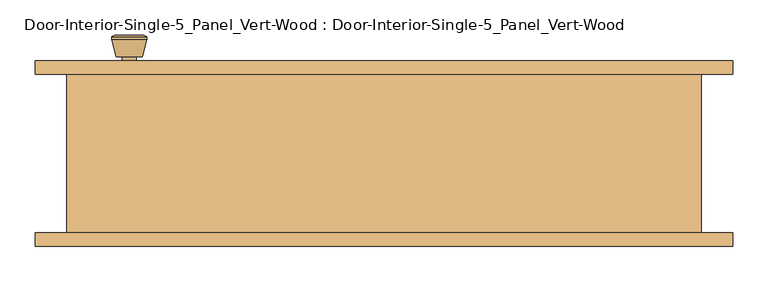
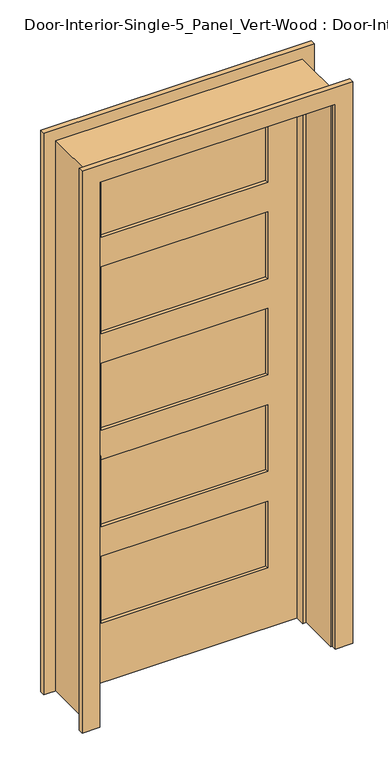
"""IFC4 building model written with IfcOpenShell, lengths in millimetres: door geometry, Door-Interior-Single-5_Panel_Vert-Wood : Door-Interior-Single-5_Panel_Vert-Wood."""

from ifc_helpers import new_model, si_unit, point, frame, frame_2d, origin, place, context, project, spatial, polyline, circle_curve, trimmed, segment, composite_curve, outline, extrude, faceted_brep, source, transform, mapped, element, save
from ifc_brep_helpers import plane_surface, cylinder_surface, revolved_surface, advanced_brep


def door_interior_single_5_panel_vert_wood_door_interior_single_0f225555(model_context):
    return source(origin(), model_context, "Body", "SolidModel", [
        advanced_brep(
        [(-361.1, 68.4, 914.4), (-351.1, 68.4, 914.4), (-371.1, 68.4, 914.4), (-340.6241324, 19.4, 914.4), (-361.1, 19.4, 914.4), (-381.5758676, 19.4, 914.4), (-336.1, 21.2278681, 914.4), (-386.1, 21.2278681, 914.4), (-336.1, 24.6915463, 914.4), (-386.1, 24.6915463, 914.4), (-342.463764, 49.4, 914.4), (-379.736236, 49.4, 914.4), (-351.1, 49.4, 914.4), (-371.1, 49.4, 914.4)],
        [
            (0, 1),
            (1, 2, circle_curve(frame((-361.1, 68.4, 914.4), z_axis=(0.0, 1.0, 0.0), x_axis=(-1.0, 0.0, 0.0)), 10.0)),
            (2, 0),
            (2, 1, circle_curve(frame((-361.1, 68.4, 914.4), z_axis=(0.0, 1.0, 0.0), x_axis=(-1.0, 0.0, 0.0)), 10.0)),
            (3, 4),
            (4, 5),
            (5, 3, circle_curve(frame((-361.1, 19.4, 914.4), z_axis=(0.0, -1.0, 0.0), x_axis=(-1.0, 0.0, 0.0)), 20.4758676)),
            (3, 5, circle_curve(frame((-361.1, 19.4, 914.4), z_axis=(0.0, -1.0, 0.0), x_axis=(-1.0, 0.0, 0.0)), 20.4758676)),
            (6, 3),
            (5, 7),
            (7, 6, circle_curve(frame((-361.1, 21.2278681, 914.4), z_axis=(0.0, -1.0, 0.0), x_axis=(-1.0, 0.0, 0.0)), 25.0)),
            (6, 7, circle_curve(frame((-361.1, 21.2278681, 914.4), z_axis=(0.0, -1.0, 0.0), x_axis=(-1.0, 0.0, 0.0)), 25.0)),
            (8, 6),
            (7, 9),
            (9, 8, circle_curve(frame((-361.1, 24.6915463, 914.4), z_axis=(0.0, -1.0, 0.0), x_axis=(-1.0, 0.0, 0.0)), 25.0)),
            (8, 9, circle_curve(frame((-361.1, 24.6915463, 914.4), z_axis=(0.0, -1.0, 0.0), x_axis=(-1.0, 0.0, 0.0)), 25.0)),
            (10, 8),
            (9, 11),
            (11, 10, circle_curve(frame((-361.1, 49.4, 914.4), z_axis=(0.0, -1.0, 0.0), x_axis=(-1.0, 0.0, 0.0)), 18.636236)),
            (10, 11, circle_curve(frame((-361.1, 49.4, 914.4), z_axis=(0.0, -1.0, 0.0), x_axis=(-1.0, 0.0, 0.0)), 18.636236)),
            (12, 10),
            (11, 13),
            (13, 12, circle_curve(frame((-361.1, 49.4, 914.4), z_axis=(0.0, -1.0, 0.0), x_axis=(-1.0, 0.0, 0.0)), 10.0)),
            (12, 13, circle_curve(frame((-361.1, 49.4, 914.4), z_axis=(0.0, -1.0, 0.0), x_axis=(-1.0, 0.0, 0.0)), 10.0)),
            (1, 12),
            (13, 2),
        ],
        [
            plane_surface(frame((-361.1, 68.4, 914.4), z_axis=(0.0, 1.0, 0.0), x_axis=(-1.0, 0.0, 0.0))),
            plane_surface(frame((-361.1, 19.4, 914.4), z_axis=(0.0, -1.0, 0.0), x_axis=(-1.0, 0.0, 0.0))),
            revolved_surface(polyline([(-381.5758676, 19.4, 914.4), (-386.1, 21.2278681, 914.4)]), (-361.1, 68.4, 914.4), (0.0, 1.0, 0.0)),
            cylinder_surface(frame((-361.1, 68.4, 914.4), z_axis=(0.0, 1.0, 0.0), x_axis=(-1.0, 0.0, 0.0)), 25.0),
            revolved_surface(polyline([(-386.1, 24.6915463, 914.4), (-379.736236, 49.4, 914.4)]), (-361.1, 68.4, 914.4), (0.0, 1.0, 0.0)),
            plane_surface(frame((-361.1, 49.4, 914.4), z_axis=(0.0, 1.0, 0.0), x_axis=(-1.0, 0.0, 0.0))),
            cylinder_surface(frame((-361.1, 68.4, 914.4), z_axis=(0.0, 1.0, 0.0), x_axis=(-1.0, 0.0, 0.0)), 10.0),
        ],
        [
            (0, [[1, 2, 3]]),
            (0, [[-3, 4, -1]]),
            (1, [[5, 6, 7]]),
            (1, [[-6, -5, 8]]),
            (2, [[9, -7, 10, 11]]),
            (2, [[-10, -8, -9, 12]]),
            (3, [[13, -11, 14, 15]]),
            (3, [[-14, -12, -13, 16]]),
            (4, [[17, -15, 18, 19]]),
            (4, [[-18, -16, -17, 20]]),
            (5, [[21, -19, 22, 23]]),
            (5, [[-22, -20, -21, 24]]),
            (6, [[25, -23, 26, -2]]),
            (6, [[-26, -24, -25, -4]]),
        ],
    ),
        extrude(outline(composite_curve([segment(trimmed(circle_curve(frame_2d((914.4, -361.1)), 30.0), [point((914.4, -391.1))], [point((914.4, -331.1))], False, "CARTESIAN"), True, "CONTINUOUS"), segment(trimmed(circle_curve(frame_2d((914.4, -361.1)), 30.0), [point((914.4, -331.1))], [point((914.4, -391.1))], False, "CARTESIAN"), True, "CONTINUOUS")], self_intersect=False)), frame((0.0, 68.4, 0.0), z_axis=(0.0, 1.0, 0.0), x_axis=(0.0, 0.0, 1.0)), (0.0, 0.0, 1.0), 6.0),
        advanced_brep(
        [(-361.1, 115.325, 914.4), (-371.1, 115.325, 914.4), (-351.1, 115.325, 914.4), (-340.6241324, 164.325, 914.4), (-381.5758676, 164.325, 914.4), (-361.1, 164.325, 914.4), (-336.1, 162.4971319, 914.4), (-386.1, 162.4971319, 914.4), (-336.1, 159.0334537, 914.4), (-386.1, 159.0334537, 914.4), (-342.463764, 134.325, 914.4), (-379.736236, 134.325, 914.4), (-351.1, 134.325, 914.4), (-371.1, 134.325, 914.4)],
        [
            (0, 1),
            (1, 2, circle_curve(frame((-361.1, 115.325, 914.4), z_axis=(0.0, -1.0, 0.0), x_axis=(-1.0, 0.0, 0.0)), 10.0)),
            (2, 0),
            (2, 1, circle_curve(frame((-361.1, 115.325, 914.4), z_axis=(0.0, -1.0, 0.0), x_axis=(-1.0, 0.0, 0.0)), 10.0)),
            (3, 4, circle_curve(frame((-361.1, 164.325, 914.4), z_axis=(0.0, 1.0, 0.0), x_axis=(-1.0, 0.0, 0.0)), 20.4758676)),
            (4, 5),
            (5, 3),
            (4, 3, circle_curve(frame((-361.1, 164.325, 914.4), z_axis=(0.0, 1.0, 0.0), x_axis=(-1.0, 0.0, 0.0)), 20.4758676)),
            (6, 7, circle_curve(frame((-361.1, 162.4971319, 914.4), z_axis=(0.0, 1.0, 0.0), x_axis=(-1.0, 0.0, 0.0)), 25.0)),
            (7, 4),
            (3, 6),
            (7, 6, circle_curve(frame((-361.1, 162.4971319, 914.4), z_axis=(0.0, 1.0, 0.0), x_axis=(-1.0, 0.0, 0.0)), 25.0)),
            (8, 9, circle_curve(frame((-361.1, 159.0334537, 914.4), z_axis=(0.0, 1.0, 0.0), x_axis=(-1.0, 0.0, 0.0)), 25.0)),
            (9, 7),
            (6, 8),
            (9, 8, circle_curve(frame((-361.1, 159.0334537, 914.4), z_axis=(0.0, 1.0, 0.0), x_axis=(-1.0, 0.0, 0.0)), 25.0)),
            (10, 11, circle_curve(frame((-361.1, 134.325, 914.4), z_axis=(0.0, 1.0, 0.0), x_axis=(-1.0, 0.0, 0.0)), 18.636236)),
            (11, 9),
            (8, 10),
            (11, 10, circle_curve(frame((-361.1, 134.325, 914.4), z_axis=(0.0, 1.0, 0.0), x_axis=(-1.0, 0.0, 0.0)), 18.636236)),
            (12, 13, circle_curve(frame((-361.1, 134.325, 914.4), z_axis=(0.0, 1.0, 0.0), x_axis=(-1.0, 0.0, 0.0)), 10.0)),
            (13, 11),
            (10, 12),
            (13, 12, circle_curve(frame((-361.1, 134.325, 914.4), z_axis=(0.0, 1.0, 0.0), x_axis=(-1.0, 0.0, 0.0)), 10.0)),
            (1, 13),
            (12, 2),
        ],
        [
            plane_surface(frame((-361.1, 115.325, 914.4), z_axis=(0.0, -1.0, 0.0), x_axis=(-1.0, 0.0, 0.0))),
            plane_surface(frame((-361.1, 164.325, 914.4), z_axis=(0.0, 1.0, 0.0), x_axis=(-1.0, 0.0, 0.0))),
            revolved_surface(polyline([(-381.5758676, 164.325, 914.4), (-386.1, 162.4971319, 914.4)]), (-361.1, 115.325, 914.4), (0.0, -1.0, 0.0)),
            cylinder_surface(frame((-361.1, 115.325, 914.4), z_axis=(0.0, -1.0, 0.0), x_axis=(-1.0, 0.0, 0.0)), 25.0),
            revolved_surface(polyline([(-386.1, 159.0334537, 914.4), (-379.736236, 134.325, 914.4)]), (-361.1, 115.325, 914.4), (0.0, -1.0, 0.0)),
            plane_surface(frame((-361.1, 134.325, 914.4), z_axis=(0.0, -1.0, 0.0), x_axis=(-1.0, 0.0, 0.0))),
            cylinder_surface(frame((-361.1, 115.325, 914.4), z_axis=(0.0, -1.0, 0.0), x_axis=(-1.0, 0.0, 0.0)), 10.0),
        ],
        [
            (0, [[1, 2, 3]]),
            (0, [[-3, 4, -1]]),
            (1, [[5, 6, 7]]),
            (1, [[8, -7, -6]]),
            (2, [[9, 10, -5, 11]]),
            (2, [[12, -11, -8, -10]]),
            (3, [[13, 14, -9, 15]]),
            (3, [[16, -15, -12, -14]]),
            (4, [[17, 18, -13, 19]]),
            (4, [[20, -19, -16, -18]]),
            (5, [[21, 22, -17, 23]]),
            (5, [[24, -23, -20, -22]]),
            (6, [[-2, 25, -21, 26]]),
            (6, [[-4, -26, -24, -25]]),
        ],
    ),
        extrude(outline(composite_curve([segment(trimmed(circle_curve(frame_2d((914.4, -361.1)), 30.0), [point((914.4, -391.1))], [point((914.4, -331.1))], False, "CARTESIAN"), True, "CONTINUOUS"), segment(trimmed(circle_curve(frame_2d((914.4, -361.1)), 30.0), [point((914.4, -331.1))], [point((914.4, -391.1))], False, "CARTESIAN"), True, "CONTINUOUS")], self_intersect=False)), frame((0.0, 109.325, 0.0), z_axis=(0.0, 1.0, 0.0), x_axis=(0.0, 0.0, 1.0)), (0.0, 0.0, 1.0), 6.0),
        faceted_brep([(450.0, 109.325, 0.0), (450.0, -115.675, 0.0), (424.6, -115.675, 0.0), (424.6, 39.475, 0.0), (411.9, 39.475, 0.0), (411.9, 74.4, 0.0), (424.6, 74.4, 0.0), (424.6, 109.325, 0.0), (450.0, 109.325, 2125.4), (450.0, -115.675, 2125.4), (-450.0, -115.675, 2125.4), (-450.0, -115.675, 0.0), (-424.6, -115.675, 0.0), (-424.6, -115.675, 2100.0), (424.6, -115.675, 2100.0), (424.6, 39.475, 2100.0), (-424.6, 39.475, 2100.0), (-424.6, 39.475, 0.0), (-411.9, 39.475, 0.0), (-411.9, 39.475, 2087.3), (411.9, 39.475, 2087.3), (411.9, 74.4, 2087.3), (-411.9, 74.4, 2087.3), (-411.9, 74.4, 0.0), (-424.6, 74.4, 0.0), (-424.6, 74.4, 2100.0), (424.6, 74.4, 2100.0), (424.6, 109.325, 2100.0), (-424.6, 109.325, 2100.0), (-424.6, 109.325, 0.0), (-450.0, 109.325, 0.0), (-450.0, 109.325, 2125.4)], [[[0, 1, 2, 3, 4, 5, 6, 7]], [[1, 0, 8, 9]], [[2, 1, 9, 10, 11, 12, 13, 14]], [[3, 2, 14, 15]], [[4, 3, 15, 16, 17, 18, 19, 20]], [[5, 4, 20, 21]], [[6, 5, 21, 22, 23, 24, 25, 26]], [[7, 6, 26, 27]], [[0, 7, 27, 28, 29, 30, 31, 8]], [[9, 8, 31, 10]], [[15, 14, 13, 16]], [[21, 20, 19, 22]], [[27, 26, 25, 28]], [[30, 29, 24, 23, 18, 17, 12, 11]], [[10, 31, 30, 11]], [[16, 13, 12, 17]], [[22, 19, 18, 23]], [[28, 25, 24, 29]]]),
        extrude(outline(polyline([(2100.0, -424.6), (0.0, -424.6), (0.0, 424.6), (2100.0, 424.6), (2100.0, -424.6)]), holes=[polyline([(1980.9375, -303.95), (1980.9375, 303.95), (1722.545, 303.95), (1722.545, -303.95), (1980.9375, -303.95)]), polyline([(490.1675, -303.95), (490.1675, 303.95), (231.775, 303.95), (231.775, -303.95), (490.1675, -303.95)]), polyline([(1235.5525, -303.95), (1235.5525, 303.95), (977.16, 303.95), (977.16, -303.95), (1235.5525, -303.95)]), polyline([(1608.245, -303.95), (1608.245, 303.95), (1349.8525, 303.95), (1349.8525, -303.95), (1608.245, -303.95)]), polyline([(862.86, -303.95), (862.86, 303.95), (604.4675, 303.95), (604.4675, -303.95), (862.86, -303.95)])]), frame((0.0, 74.4, 0.0), z_axis=(0.0, 1.0, 0.0), x_axis=(0.0, 0.0, 1.0)), (0.0, 0.0, 1.0), 34.925),
        extrude(outline(polyline([(303.95, 86.0416667), (-303.95, 86.0416667), (-303.95, 97.6833333), (303.95, 97.6833333), (303.95, 86.0416667)])), frame((0.0, 0.0, 1722.545), z_axis=(0.0, 0.0, 1.0), x_axis=(1.0, 0.0, 0.0)), (0.0, 0.0, 1.0), 258.3925),
        extrude(outline(polyline([(303.95, 86.0416667), (-303.95, 86.0416667), (-303.95, 97.6833333), (303.95, 97.6833333), (303.95, 86.0416667)])), frame((0.0, 0.0, 1349.8525), z_axis=(0.0, 0.0, 1.0), x_axis=(1.0, 0.0, 0.0)), (0.0, 0.0, 1.0), 258.3925),
        extrude(outline(polyline([(303.95, 86.0416667), (-303.95, 86.0416667), (-303.95, 97.6833333), (303.95, 97.6833333), (303.95, 86.0416667)])), frame((0.0, 0.0, 604.4675), z_axis=(0.0, 0.0, 1.0), x_axis=(1.0, 0.0, 0.0)), (0.0, 0.0, 1.0), 258.3925),
        extrude(outline(polyline([(303.95, 86.0416667), (-303.95, 86.0416667), (-303.95, 97.6833333), (303.95, 97.6833333), (303.95, 86.0416667)])), frame((0.0, 0.0, 231.775), z_axis=(0.0, 0.0, 1.0), x_axis=(1.0, 0.0, 0.0)), (0.0, 0.0, 1.0), 258.3925),
        extrude(outline(polyline([(303.95, 86.0416667), (-303.95, 86.0416667), (-303.95, 97.6833333), (303.95, 97.6833333), (303.95, 86.0416667)])), frame((0.0, 0.0, 977.16), z_axis=(0.0, 0.0, 1.0), x_axis=(1.0, 0.0, 0.0)), (0.0, 0.0, 1.0), 258.3925),
        extrude(outline(polyline([(0.0, 430.95), (0.0, 494.45), (2169.85, 494.45), (2169.85, -494.45), (0.0, -494.45), (0.0, -430.95), (2106.35, -430.95), (2106.35, 430.95), (0.0, 430.95)])), frame((0.0, 109.325, 0.0), z_axis=(0.0, 1.0, 0.0), x_axis=(0.0, 0.0, 1.0)), (0.0, 0.0, 1.0), 19.05),
        extrude(outline(polyline([(0.0, 430.95), (0.0, 494.45), (2169.85, 494.45), (2169.85, -494.45), (0.0, -494.45), (0.0, -430.95), (2106.35, -430.95), (2106.35, 430.95), (0.0, 430.95)])), frame((0.0, -134.725, 0.0), z_axis=(0.0, 1.0, 0.0), x_axis=(0.0, 0.0, 1.0)), (0.0, 0.0, 1.0), 19.05),
    ])


if __name__ == "__main__":
    model = new_model("IFC4")
    model_context = context("Model", 3, world=origin())
    ifc_project = project(units=[si_unit("LENGTHUNIT", "METRE", prefix="MILLI")], contexts=[model_context])
    site = spatial("IfcSite", under=ifc_project)
    building = spatial("IfcBuilding", under=site)
    placement = place(None, origin())
    door_interior_single_5_panel_vert_wood_door_interior_single_shape = door_interior_single_5_panel_vert_wood_door_interior_single_0f225555(model_context)
    element("IfcDoor", 1, ObjectType="Door-Interior-Single-5_Panel_Vert-Wood : Door-Interior-Single-5_Panel_Vert-Wood", at=placement, inside=building, context=model_context, shape_type="MappedRepresentation", body=[
        mapped(door_interior_single_5_panel_vert_wood_door_interior_single_shape, transform((0.0, 0.0, 0.0), x_axis=(1.0, 0.0, 0.0), y_axis=(0.0, 1.0, 0.0), z_axis=(0.0, 0.0, 1.0))),
    ])
    save(model, "model.ifc")

# Revit data of these elements
# Type "Door-Interior-Single-5_Panel_Vert-Wood : Door-Interior-Single-5_Panel_Vert-Wood"
#   Type Mark = "46"
#   Assembly Code = "C1020300"
#   Analytic Construction = "Wooden"
#   Top Rail = 119.063 mm
#   Thickness = 34.925 mm
#   Thermal Resistance (R) = 0.455703 (m²·K)/W
#   Swing Angle [instance default] = 90.00°
#   Stiles = 120.65 mm
#   Rough Width = 900 mm
#   Rough Height = 2125.4 mm
#   Intermediate Rail = 114.3 mm
#   Height = 2100 mm
#   Width = 849.2 mm
#   Heat Transfer Coefficient (U) = 2.19465 W/(m²·K)
#   Bottom Rail = 231.775 mm
#   Trim Material = Cherry
#   Panel Material = Cherry
#   Frame Material = Cherry
#   Door Handle Material = Aluminum
#   Visual Light Transmittance = 0
#   Solar Heat Gain Coefficient = 0
#   Wall Closure = (empty or 0)
#   Function = (empty or 0)
# Element 1 (IfcDoor, "Door-Interior-Single-5_Panel_Vert-Wood : Door-Interior-Single-5_Panel_Vert-Wood")
#   Materials on its faces: "Cherry", "Aluminum"
# Materials
#   "Cherry": class "Wood", colour RGB 226 177 128, transparency 0, Description = "Prunus Serotina", Cost = 0
#   "Aluminum": class "Metal", colour RGB 247 247 247, transparency 0, Description = "Aluminum 6061", Cost = 0
